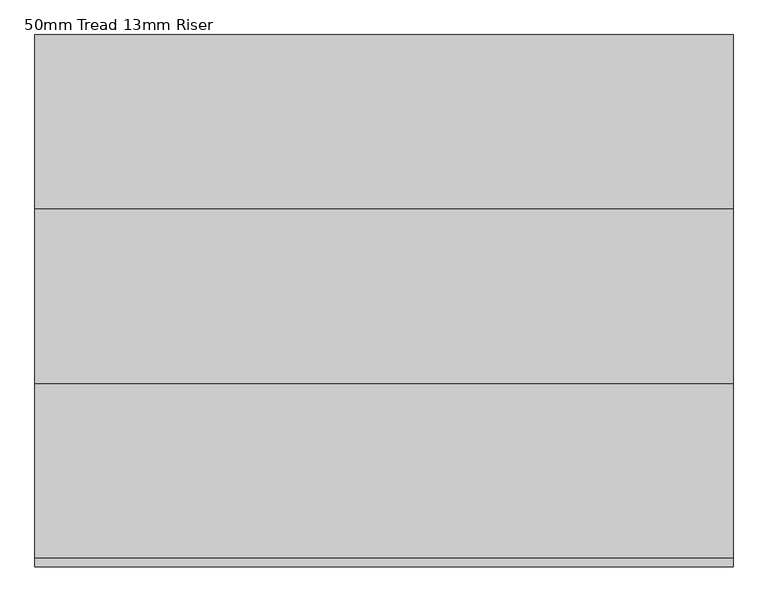
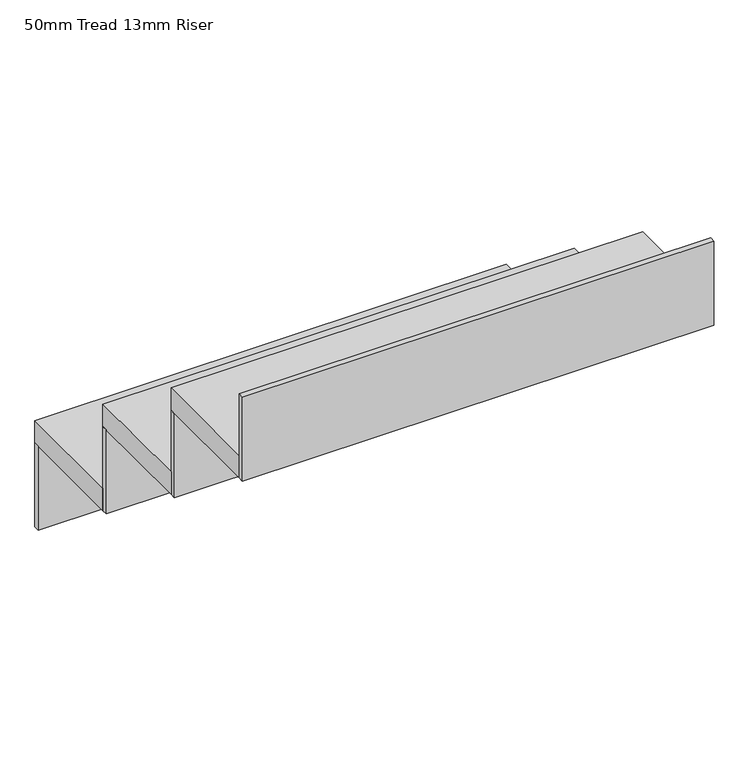
"""IFC4 building model written with IfcOpenShell, lengths in millimetres: stair flight geometry, 50mm Tread 13mm Riser."""

from ifc_helpers import new_model, si_unit, frame, origin, place, context, project, spatial, polyline, outline, extrude, source, transform, mapped, element, save


def stair_flight_50mm_tread_13mm_riser_a88b1a6b(model_context):
    return source(origin(), model_context, "Body", "SweptSolid", [
        extrude(outline(polyline([(-10477.6052721, -2511.0618509), (-10477.6052721, -2498.5618509), (-9477.5794909, -2498.5618509), (-9477.5794909, -2511.0618509), (-10477.6052721, -2511.0618509)])), frame((0.0, 0.0, 4468.2117647), z_axis=(0.0, 0.0, 1.0), x_axis=(1.0, 0.0, 0.0)), (0.0, 0.0, 1.0), 188.2588235),
        extrude(outline(polyline([(-9477.5794909, -2748.5618509), (-10477.6052721, -2748.5618509), (-10477.6052721, -2498.5618509), (-9477.5794909, -2498.5618509), (-9477.5794909, -2748.5618509)])), frame((0.0, 0.0, 4656.4705882), z_axis=(0.0, 0.0, 1.0), x_axis=(1.0, 0.0, 0.0)), (0.0, 0.0, 1.0), 50.0),
        extrude(outline(polyline([(-10477.6052721, -2761.0618509), (-10477.6052721, -2748.5618509), (-9477.5794909, -2748.5618509), (-9477.5794909, -2761.0618509), (-10477.6052721, -2761.0618509)])), frame((0.0, 0.0, 4656.4705882), z_axis=(0.0, 0.0, 1.0), x_axis=(1.0, 0.0, 0.0)), (0.0, 0.0, 1.0), 188.2588235),
        extrude(outline(polyline([(-9477.5794909, -2998.5618509), (-10477.6052721, -2998.5618509), (-10477.6052721, -2748.5618509), (-9477.5794909, -2748.5618509), (-9477.5794909, -2998.5618509)])), frame((0.0, 0.0, 4844.7294118), z_axis=(0.0, 0.0, 1.0), x_axis=(1.0, 0.0, 0.0)), (0.0, 0.0, 1.0), 50.0),
        extrude(outline(polyline([(-10477.6052721, -3011.0618509), (-10477.6052721, -2998.5618509), (-9477.5794909, -2998.5618509), (-9477.5794909, -3011.0618509), (-10477.6052721, -3011.0618509)])), frame((0.0, 0.0, 4844.7294118), z_axis=(0.0, 0.0, 1.0), x_axis=(1.0, 0.0, 0.0)), (0.0, 0.0, 1.0), 188.2588235),
        extrude(outline(polyline([(-10477.6052721, -3261.0618509), (-10477.6052721, -3248.5618509), (-9477.5794909, -3248.5618509), (-9477.5794909, -3261.0618509), (-10477.6052721, -3261.0618509)])), frame((0.0, 0.0, 5032.9882353), z_axis=(0.0, 0.0, 1.0), x_axis=(1.0, 0.0, 0.0)), (0.0, 0.0, 1.0), 188.2588235),
        extrude(outline(polyline([(-9477.5794909, -3248.5618509), (-10477.6052721, -3248.5618509), (-10477.6052721, -2998.5618509), (-9477.5794909, -2998.5618509), (-9477.5794909, -3248.5618509)])), frame((0.0, 0.0, 5032.9882353), z_axis=(0.0, 0.0, 1.0), x_axis=(1.0, 0.0, 0.0)), (0.0, 0.0, 1.0), 50.0),
    ])


if __name__ == "__main__":
    model = new_model("IFC4")
    model_context = context("Model", 3, world=origin())
    ifc_project = project(units=[si_unit("LENGTHUNIT", "METRE", prefix="MILLI")], contexts=[model_context])
    site = spatial("IfcSite", under=ifc_project)
    building = spatial("IfcBuilding", under=site)
    placement = place(None, origin())
    stair_flight_50mm_tread_13mm_riser_shape = stair_flight_50mm_tread_13mm_riser_a88b1a6b(model_context)
    element("IfcStairFlight", 1, ObjectType="50mm Tread 13mm Riser", at=placement, inside=building, context=model_context, shape_type="MappedRepresentation", body=[
        mapped(stair_flight_50mm_tread_13mm_riser_shape, transform((0.0, 0.0, 0.0), x_axis=(1.0, 0.0, 0.0), y_axis=(0.0, 1.0, 0.0), z_axis=(0.0, 0.0, 1.0))),
    ])
    save(model, "model.ifc")
